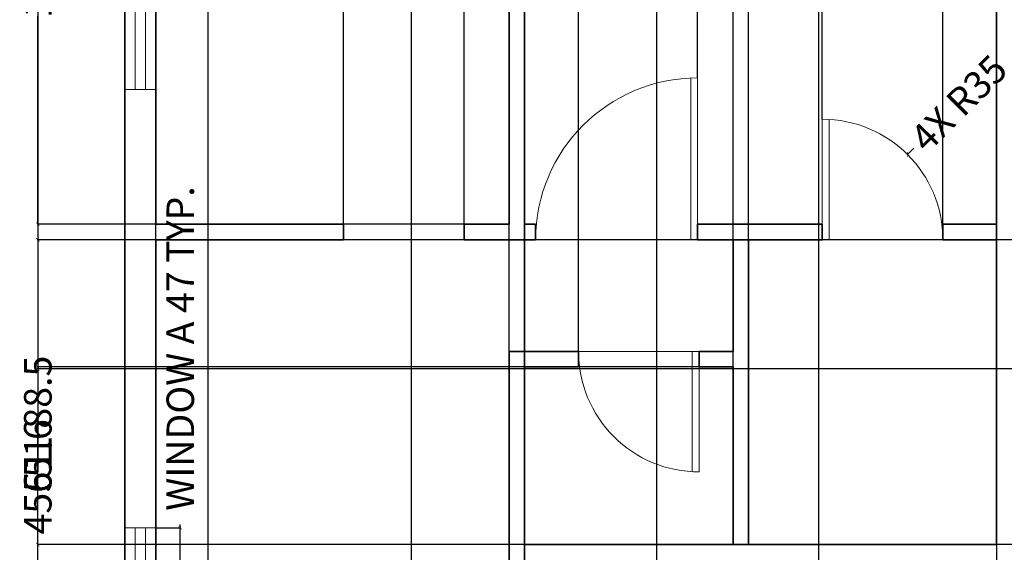
# Model space of a CAD drawing. Units: inches. Extents: x 878 to 1443, y 634 to 1188.
# Tile 2 of 5: x 878 to 1164, y 878 to 1033. Entities that reach past the tile are written whole.
import ezdxf

# ---------------------------------------------------------------- set-up
doc = ezdxf.new("R2010")
doc.units = ezdxf.units.IN
doc.header["$MEASUREMENT"] = 0
doc.layers.add('A-ANNO-DIMS', color=2, linetype='Continuous', lineweight=18)
doc.layers.add('A-WALL', color=7, linetype='Continuous', lineweight=35)
doc.layers.add('A-DOOR', color=41, linetype='Continuous', lineweight=18, true_color=0xf4ee51)
doc.layers.add('A-GLAZ', color=152, linetype='Continuous', lineweight=18, true_color=0x2776bb)
doc.styles.get("Standard").update_dxf_attribs({"font": 'arial.ttf'})
doc.dimstyles.get("Standard").update_dxf_attribs({"dimtxt": 8, "dimasz": 1, "dimexe": 0.18, "dimexo": 0.0625, "dimgap": 0.09, "dimtad": 0, "dimdec": 4, "dimzin": 0, "dimdsep": 46, "dimlunit": 3, "dimtxsty": 'Standard', "dimblk": 'ARCHTICK', "dimcen": 0.09, "dimclrd": 6, "dimclre": 5, "dimclrt": 140, "dimadec": 0, "dimazin": 0, "dimtfac": 1, "dimtdec": 4, "dimtofl": 0, "dimtmove": 0, "dimatfit": 3, "dimfxl": 1, "dimtolj": 1, "dimtzin": 0, "dimarcsym": 0})

# ---------------------------------------------------------------- blocks, each defined once
blk = doc.blocks.new('WIN-47IN')
for p, q in [((9, 47), (0, 47)), ((0, 47), (0, 0)), ((3, 0), (3, 47)), ((6, 0), (6, 47)), ((9, 0), (9, 47)), ((0, 0), (9, 0))]:
    blk.add_line(p, q)
blk = doc.blocks.new('DOOR-47IN')
for p, q in [((0, 47), (0, 0)), ((0, 2), (46.96, 2)), ((0, 0), (47, 0))]:
    blk.add_line(p, q)
blk.add_arc((0, 0), 47, 0, 90)
blk = doc.blocks.new('DOOR-35IN')
for p, q in [((0, 35), (0, 0)), ((2, 34.94), (2, 0)), ((0, 0), (35, 0))]:
    blk.add_line(p, q)
blk.add_arc((0, 0), 35, 360, 90)
blk = doc.blocks.new('_ArchTick')
at = {"color": 0, "linetype": 'ByBlock', "const_width": 0.15}
blk.add_lwpolyline([(-0.5, -0.5), (0.5, 0.5)], dxfattribs=at)
blk = doc.blocks.new('*D9')
at = {"layer": 'A-ANNO-DIMS', "color": 6, "lineweight": -2, "transparency": 16777216}
for p, q in [((924.95, 885.33), (924.95, 886.33)), ((924.95, 838.33), (924.95, 885.33))]:
    blk.add_line(p, q, dxfattribs=at)
at = {"layer": 'A-ANNO-DIMS', "color": 5, "lineweight": -2, "transparency": 16777216}
for p, q in [((917.96, 885.33), (925.13, 885.33)), ((917.96, 838.33), (925.13, 838.33))]:
    blk.add_line(p, q, dxfattribs=at)
at = {"layer": 'Defpoints', "color": 0, "lineweight": -2, "transparency": 16777216}
for p in [(917.9, 885.33), (924.95, 885.33), (917.9, 838.33)]:
    blk.add_point(p, dxfattribs=at)
at = {"layer": 'A-ANNO-DIMS', "color": 6, "lineweight": -2, "transparency": 16777216}
for p, rotation in [((924.95, 885.33), 90), ((924.95, 838.33), 270)]:
    blk.add_blockref('_ArchTick', p, dxfattribs=dict(at, rotation=rotation))
at = {"layer": 'A-ANNO-DIMS', "color": 140, "transparency": 16777216, "insert": (924.95, 937.4), "char_height": 8, "attachment_point": 5, "rotation": 90}
blk.add_mtext('\\A1;WINDOW A 47 TYP.', dxfattribs=at)
blk = doc.blocks.new('*D22')
at = {"layer": 'A-ANNO-DIMS', "color": 5, "lineweight": -2, "transparency": 16777216}
for p, q in [((908.84, 1120.47), (883.41, 1120.47)), ((908.84, 664.47), (883.41, 664.47))]:
    blk.add_line(p, q, dxfattribs=at)
at = {"layer": 'A-ANNO-DIMS', "color": 6, "lineweight": -2, "transparency": 16777216}
for p, q in [((883.59, 1120.47), (883.59, 901.56)), ((883.59, 664.47), (883.59, 883.38))]:
    blk.add_line(p, q, dxfattribs=at)
at = {"layer": 'Defpoints', "color": 0, "lineweight": -2, "transparency": 16777216}
for p in [(883.59, 1120.47), (908.9, 1120.47), (908.9, 664.47)]:
    blk.add_point(p, dxfattribs=at)
at = {"layer": 'A-ANNO-DIMS', "color": 6, "lineweight": -2, "transparency": 16777216}
for p, rotation in [((883.59, 1120.47), 90), ((883.59, 664.47), 270)]:
    blk.add_blockref('_ArchTick', p, dxfattribs=dict(at, rotation=rotation))
at = {"layer": 'A-ANNO-DIMS', "color": 140, "transparency": 16777216, "insert": (883.59, 892.47), "char_height": 8, "attachment_point": 5, "rotation": 90}
blk.add_mtext('\\A1;456', dxfattribs=at)
blk = doc.blocks.new('*D33')
at = {"layer": 'A-ANNO-DIMS', "color": 5, "lineweight": -2, "transparency": 16777216}
for p, q in [((917.9, 760.53), (917.9, 1145.96)), ((1020.4, 760.53), (1020.4, 1145.96))]:
    blk.add_line(p, q, dxfattribs=at)
at = {"layer": 'A-ANNO-DIMS', "color": 6, "lineweight": -2, "transparency": 16777216}
for p, q in [((917.9, 1145.78), (955.91, 1145.78)), ((1020.4, 1145.78), (982.39, 1145.78))]:
    blk.add_line(p, q, dxfattribs=at)
at = {"layer": 'Defpoints', "color": 0, "lineweight": -2, "transparency": 16777216}
for p in [(1020.4, 1145.78), (917.9, 760.47), (1020.4, 760.47)]:
    blk.add_point(p, dxfattribs=at)
at = {"layer": 'A-ANNO-DIMS', "color": 6, "lineweight": -2, "transparency": 16777216, "rotation": 180}
blk.add_blockref('_ArchTick', (917.9, 1145.78), dxfattribs=at)
at = {"layer": 'A-ANNO-DIMS', "color": 6, "lineweight": -2, "transparency": 16777216}
blk.add_blockref('_ArchTick', (1020.4, 1145.78), dxfattribs=at)
at = {"layer": 'A-ANNO-DIMS', "color": 140, "transparency": 16777216, "insert": (969.15, 1145.78), "char_height": 8, "attachment_point": 5}
blk.add_mtext('\\A1;102.5', dxfattribs=at)
blk = doc.blocks.new('*D34')
at = {"layer": 'A-ANNO-DIMS', "color": 5, "lineweight": -2, "transparency": 16777216}
for p, q in [((1024.9, 1111.41), (1024.9, 638.98)), ((1161.9, 1111.41), (1161.9, 638.98))]:
    blk.add_line(p, q, dxfattribs=at)
at = {"layer": 'A-ANNO-DIMS', "color": 6, "lineweight": -2, "transparency": 16777216}
for p, q in [((1024.9, 639.16), (1084.85, 639.16)), ((1161.9, 639.16), (1101.95, 639.16))]:
    blk.add_line(p, q, dxfattribs=at)
at = {"layer": 'Defpoints', "color": 0, "lineweight": -2, "transparency": 16777216}
for p in [(1024.9, 1111.47), (1161.9, 1111.47), (1161.9, 639.16)]:
    blk.add_point(p, dxfattribs=at)
at = {"layer": 'A-ANNO-DIMS', "color": 6, "lineweight": -2, "transparency": 16777216, "rotation": 180}
blk.add_blockref('_ArchTick', (1024.9, 639.16), dxfattribs=at)
at = {"layer": 'A-ANNO-DIMS', "color": 6, "lineweight": -2, "transparency": 16777216}
blk.add_blockref('_ArchTick', (1161.9, 639.16), dxfattribs=at)
at = {"layer": 'A-ANNO-DIMS', "color": 140, "transparency": 16777216, "insert": (1093.4, 639.16), "char_height": 8, "attachment_point": 5}
blk.add_mtext('\\A1;137', dxfattribs=at)
blk = doc.blocks.new('*D36')
at = {"layer": 'A-ANNO-DIMS', "color": 5, "lineweight": -2, "transparency": 16777216}
for p, q in [((1020.34, 1111.47), (883.41, 1111.47)), ((1020.34, 973.47), (883.41, 973.47))]:
    blk.add_line(p, q, dxfattribs=at)
at = {"layer": 'A-ANNO-DIMS', "color": 6, "lineweight": -2, "transparency": 16777216}
for p, q in [((883.59, 1111.47), (883.59, 1051.03)), ((883.59, 973.47), (883.59, 1033.91))]:
    blk.add_line(p, q, dxfattribs=at)
at = {"layer": 'Defpoints', "color": 0, "lineweight": -2, "transparency": 16777216}
for p in [(1020.4, 1111.47), (883.59, 973.47), (1020.4, 973.47)]:
    blk.add_point(p, dxfattribs=at)
at = {"layer": 'A-ANNO-DIMS', "color": 6, "lineweight": -2, "transparency": 16777216}
for p, rotation in [((883.59, 1111.47), 90), ((883.59, 973.47), 270)]:
    blk.add_blockref('_ArchTick', p, dxfattribs=dict(at, rotation=rotation))
at = {"layer": 'A-ANNO-DIMS', "color": 140, "transparency": 16777216, "insert": (883.59, 1042.47), "char_height": 8, "attachment_point": 5, "rotation": 90}
blk.add_mtext('\\A1;138', dxfattribs=at)
blk = doc.blocks.new('*D37')
at = {"layer": 'A-ANNO-DIMS', "color": 5, "lineweight": -2, "transparency": 16777216}
for p, q in [((1403.84, 968.97), (883.41, 968.97)), ((1403.84, 880.47), (883.41, 880.47))]:
    blk.add_line(p, q, dxfattribs=at)
at = {"layer": 'A-ANNO-DIMS', "color": 6, "lineweight": -2, "transparency": 16777216}
for p, q in [((883.59, 968.97), (883.59, 935.24)), ((883.59, 880.47), (883.59, 914.2))]:
    blk.add_line(p, q, dxfattribs=at)
at = {"layer": 'Defpoints', "color": 0, "lineweight": -2, "transparency": 16777216}
for p in [(1403.9, 968.97), (883.59, 880.47), (1403.9, 880.47)]:
    blk.add_point(p, dxfattribs=at)
at = {"layer": 'A-ANNO-DIMS', "color": 6, "lineweight": -2, "transparency": 16777216}
for p, rotation in [((883.59, 968.97), 90), ((883.59, 880.47), 270)]:
    blk.add_blockref('_ArchTick', p, dxfattribs=dict(at, rotation=rotation))
at = {"layer": 'A-ANNO-DIMS', "color": 140, "transparency": 16777216, "insert": (883.59, 924.72), "char_height": 8, "attachment_point": 5, "rotation": 90}
blk.add_mtext('\\A1;88.5', dxfattribs=at)
blk = doc.blocks.new('*D39')
at = {"layer": 'A-ANNO-DIMS', "color": 5, "lineweight": -2, "transparency": 16777216}
for p, q in [((1024.9, 880.53), (1024.9, 1145.96)), ((1085.4, 880.53), (1085.4, 1145.96))]:
    blk.add_line(p, q, dxfattribs=at)
at = {"layer": 'A-ANNO-DIMS', "color": 6, "lineweight": -2, "transparency": 16777216}
for p, q in [((1024.9, 1145.78), (1044.62, 1145.78)), ((1085.4, 1145.78), (1065.68, 1145.78))]:
    blk.add_line(p, q, dxfattribs=at)
at = {"layer": 'Defpoints', "color": 0, "lineweight": -2, "transparency": 16777216}
for p in [(1085.4, 1145.78), (1024.9, 880.47), (1085.4, 880.47)]:
    blk.add_point(p, dxfattribs=at)
at = {"layer": 'A-ANNO-DIMS', "color": 6, "lineweight": -2, "transparency": 16777216, "rotation": 180}
blk.add_blockref('_ArchTick', (1024.9, 1145.78), dxfattribs=at)
at = {"layer": 'A-ANNO-DIMS', "color": 6, "lineweight": -2, "transparency": 16777216}
blk.add_blockref('_ArchTick', (1085.4, 1145.78), dxfattribs=at)
at = {"layer": 'A-ANNO-DIMS', "color": 140, "transparency": 16777216, "insert": (1055.15, 1145.78), "char_height": 8, "attachment_point": 5}
blk.add_mtext('\\A1;60.5', dxfattribs=at)
blk = doc.blocks.new('*D40')
at = {"layer": 'A-ANNO-DIMS', "color": 5, "lineweight": -2, "transparency": 16777216}
for p, q in [((1089.9, 880.53), (1089.9, 1145.96)), ((1161.9, 880.53), (1161.9, 1145.96))]:
    blk.add_line(p, q, dxfattribs=at)
at = {"layer": 'A-ANNO-DIMS', "color": 6, "lineweight": -2, "transparency": 16777216}
for p, q in [((1089.9, 1145.78), (1120.15, 1145.78)), ((1161.9, 1145.78), (1131.64, 1145.78))]:
    blk.add_line(p, q, dxfattribs=at)
at = {"layer": 'Defpoints', "color": 0, "lineweight": -2, "transparency": 16777216}
for p in [(1161.9, 1145.78), (1089.9, 880.47), (1161.9, 880.47)]:
    blk.add_point(p, dxfattribs=at)
at = {"layer": 'A-ANNO-DIMS', "color": 6, "lineweight": -2, "transparency": 16777216, "rotation": 180}
blk.add_blockref('_ArchTick', (1089.9, 1145.78), dxfattribs=at)
at = {"layer": 'A-ANNO-DIMS', "color": 6, "lineweight": -2, "transparency": 16777216}
blk.add_blockref('_ArchTick', (1161.9, 1145.78), dxfattribs=at)
at = {"layer": 'A-ANNO-DIMS', "color": 140, "transparency": 16777216, "insert": (1125.9, 1145.78), "char_height": 8, "attachment_point": 5}
blk.add_mtext('\\A1;72', dxfattribs=at)
blk = doc.blocks.new('*D42')
at = {"layer": 'A-ANNO-DIMS', "color": 5, "lineweight": -2, "transparency": 16777216}
for p, q in [((1085.34, 932.07), (883.41, 932.07)), ((1085.34, 880.47), (883.41, 880.47))]:
    blk.add_line(p, q, dxfattribs=at)
at = {"layer": 'A-ANNO-DIMS', "color": 6, "lineweight": -2, "transparency": 16777216}
for p, q in [((883.59, 932.07), (883.59, 916.75)), ((883.59, 880.47), (883.59, 895.79))]:
    blk.add_line(p, q, dxfattribs=at)
at = {"layer": 'Defpoints', "color": 0, "lineweight": -2, "transparency": 16777216}
for p in [(883.59, 932.07), (1085.4, 932.07), (1085.4, 880.47)]:
    blk.add_point(p, dxfattribs=at)
at = {"layer": 'A-ANNO-DIMS', "color": 6, "lineweight": -2, "transparency": 16777216}
for p, rotation in [((883.59, 932.07), 90), ((883.59, 880.47), 270)]:
    blk.add_blockref('_ArchTick', p, dxfattribs=dict(at, rotation=rotation))
at = {"layer": 'A-ANNO-DIMS', "color": 140, "transparency": 16777216, "insert": (883.59, 906.27), "char_height": 8, "attachment_point": 5, "rotation": 90}
blk.add_mtext('\\A1;51.6', dxfattribs=at)
blk = doc.blocks.new('*D43')
at = {"layer": 'A-ANNO-DIMS', "color": 5, "lineweight": -2, "transparency": 16777216}
for p, q in [((1327.34, 931.47), (883.41, 931.47)), ((1327.34, 880.47), (883.41, 880.47))]:
    blk.add_line(p, q, dxfattribs=at)
at = {"layer": 'A-ANNO-DIMS', "color": 6, "lineweight": -2, "transparency": 16777216}
for p, q in [((883.59, 931.47), (883.59, 911.02)), ((883.59, 880.47), (883.59, 900.92))]:
    blk.add_line(p, q, dxfattribs=at)
at = {"layer": 'Defpoints', "color": 0, "lineweight": -2, "transparency": 16777216}
for p in [(883.59, 931.47), (1327.4, 931.47), (1327.4, 880.47)]:
    blk.add_point(p, dxfattribs=at)
at = {"layer": 'A-ANNO-DIMS', "color": 6, "lineweight": -2, "transparency": 16777216}
for p, rotation in [((883.59, 931.47), 90), ((883.59, 880.47), 270)]:
    blk.add_blockref('_ArchTick', p, dxfattribs=dict(at, rotation=rotation))
at = {"layer": 'A-ANNO-DIMS', "color": 140, "transparency": 16777216, "insert": (883.59, 905.97), "char_height": 8, "attachment_point": 5, "rotation": 90}
blk.add_mtext('\\A1;51', dxfattribs=at)
blk = doc.blocks.new('*D44')
at = {"layer": 'A-ANNO-DIMS', "color": 5, "lineweight": -2, "transparency": 16777216}
for p, q in [((917.9, 751.53), (917.9, 1145.96)), ((933.09, 751.53), (933.09, 1145.96))]:
    blk.add_line(p, q, dxfattribs=at)
at = {"layer": 'A-ANNO-DIMS', "color": 6, "lineweight": -2, "transparency": 16777216}
for p, q in [((917.9, 1145.78), (933.09, 1145.78)), ((933.09, 1145.78), (934.09, 1145.78))]:
    blk.add_line(p, q, dxfattribs=at)
at = {"layer": 'Defpoints', "color": 0, "lineweight": -2, "transparency": 16777216}
for p in [(933.09, 1145.78), (917.9, 751.47), (933.09, 751.47)]:
    blk.add_point(p, dxfattribs=at)
at = {"layer": 'A-ANNO-DIMS', "color": 6, "lineweight": -2, "transparency": 16777216, "rotation": 180}
blk.add_blockref('_ArchTick', (917.9, 1145.78), dxfattribs=at)
at = {"layer": 'A-ANNO-DIMS', "color": 6, "lineweight": -2, "transparency": 16777216}
blk.add_blockref('_ArchTick', (933.09, 1145.78), dxfattribs=at)
at = {"layer": 'A-ANNO-DIMS', "color": 140, "transparency": 16777216, "insert": (950.4, 1145.78), "char_height": 8, "attachment_point": 5}
blk.add_mtext('\\A1;15.187', dxfattribs=at)
blk = doc.blocks.new('*D45')
at = {"layer": 'A-ANNO-DIMS', "color": 5, "lineweight": -2, "transparency": 16777216}
for p, q in [((992.09, 751.53), (992.09, 1145.96)), ((1063.3, 751.53), (1063.3, 1145.96))]:
    blk.add_line(p, q, dxfattribs=at)
at = {"layer": 'A-ANNO-DIMS', "color": 6, "lineweight": -2, "transparency": 16777216}
for p, q in [((992.09, 1145.78), (1014.18, 1145.78)), ((1063.3, 1145.78), (1041.21, 1145.78))]:
    blk.add_line(p, q, dxfattribs=at)
at = {"layer": 'Defpoints', "color": 0, "lineweight": -2, "transparency": 16777216}
for p in [(1063.3, 1145.78), (992.09, 751.47), (1063.3, 751.47)]:
    blk.add_point(p, dxfattribs=at)
at = {"layer": 'A-ANNO-DIMS', "color": 6, "lineweight": -2, "transparency": 16777216, "rotation": 180}
blk.add_blockref('_ArchTick', (992.09, 1145.78), dxfattribs=at)
at = {"layer": 'A-ANNO-DIMS', "color": 6, "lineweight": -2, "transparency": 16777216}
blk.add_blockref('_ArchTick', (1063.3, 1145.78), dxfattribs=at)
at = {"layer": 'A-ANNO-DIMS', "color": 140, "transparency": 16777216, "insert": (1027.69, 1145.78), "char_height": 8, "attachment_point": 5}
blk.add_mtext('\\A1;71.22', dxfattribs=at)
blk = doc.blocks.new('*D46')
at = {"layer": 'A-ANNO-DIMS', "color": 5, "lineweight": -2, "transparency": 16777216}
for p, q in [((1110.3, 751.53), (1110.3, 1145.96)), ((1172.39, 751.53), (1172.39, 1145.96))]:
    blk.add_line(p, q, dxfattribs=at)
at = {"layer": 'A-ANNO-DIMS', "color": 6, "lineweight": -2, "transparency": 16777216}
for p, q in [((1110.3, 1145.78), (1127.73, 1145.78)), ((1172.39, 1145.78), (1154.96, 1145.78))]:
    blk.add_line(p, q, dxfattribs=at)
at = {"layer": 'Defpoints', "color": 0, "lineweight": -2, "transparency": 16777216}
for p in [(1172.39, 1145.78), (1110.3, 751.47), (1172.39, 751.47)]:
    blk.add_point(p, dxfattribs=at)
at = {"layer": 'A-ANNO-DIMS', "color": 6, "lineweight": -2, "transparency": 16777216, "rotation": 180}
blk.add_blockref('_ArchTick', (1110.3, 1145.78), dxfattribs=at)
at = {"layer": 'A-ANNO-DIMS', "color": 6, "lineweight": -2, "transparency": 16777216}
blk.add_blockref('_ArchTick', (1172.39, 1145.78), dxfattribs=at)
at = {"layer": 'A-ANNO-DIMS', "color": 140, "transparency": 16777216, "insert": (1141.35, 1145.78), "char_height": 8, "attachment_point": 5}
blk.add_mtext('\\A1;62.08', dxfattribs=at)
blk = doc.blocks.new('*D49')
at = {"layer": 'A-ANNO-DIMS', "color": 5, "lineweight": -2, "transparency": 16777216}
for p, q in [((917.9, 973.53), (917.9, 1145.96)), ((972.37, 973.53), (972.37, 1145.96))]:
    blk.add_line(p, q, dxfattribs=at)
at = {"layer": 'A-ANNO-DIMS', "color": 6, "lineweight": -2, "transparency": 16777216}
for p, q in [((917.9, 1145.78), (931.54, 1145.78)), ((972.37, 1145.78), (958.72, 1145.78))]:
    blk.add_line(p, q, dxfattribs=at)
at = {"layer": 'Defpoints', "color": 0, "lineweight": -2, "transparency": 16777216}
for p in [(972.37, 1145.78), (917.9, 973.47), (972.37, 973.47)]:
    blk.add_point(p, dxfattribs=at)
at = {"layer": 'A-ANNO-DIMS', "color": 6, "lineweight": -2, "transparency": 16777216, "rotation": 180}
blk.add_blockref('_ArchTick', (917.9, 1145.78), dxfattribs=at)
at = {"layer": 'A-ANNO-DIMS', "color": 6, "lineweight": -2, "transparency": 16777216}
blk.add_blockref('_ArchTick', (972.37, 1145.78), dxfattribs=at)
at = {"layer": 'A-ANNO-DIMS', "color": 140, "transparency": 16777216, "insert": (945.13, 1145.78), "char_height": 8, "attachment_point": 5}
blk.add_mtext('\\A1;54.47', dxfattribs=at)
blk = doc.blocks.new('*D50')
at = {"layer": 'A-ANNO-DIMS', "color": 5, "lineweight": -2, "transparency": 16777216}
for p, q in [((972.37, 973.53), (972.37, 1145.96)), ((1007.37, 973.53), (1007.37, 1145.96))]:
    blk.add_line(p, q, dxfattribs=at)
at = {"layer": 'A-ANNO-DIMS', "color": 6, "lineweight": -2, "transparency": 16777216}
for p, q in [((972.37, 1145.78), (984.02, 1145.78)), ((1007.37, 1145.78), (995.71, 1145.78))]:
    blk.add_line(p, q, dxfattribs=at)
at = {"layer": 'Defpoints', "color": 0, "lineweight": -2, "transparency": 16777216}
for p in [(1007.37, 1145.78), (972.37, 973.47), (1007.37, 973.47)]:
    blk.add_point(p, dxfattribs=at)
at = {"layer": 'A-ANNO-DIMS', "color": 6, "lineweight": -2, "transparency": 16777216, "rotation": 180}
blk.add_blockref('_ArchTick', (972.37, 1145.78), dxfattribs=at)
at = {"layer": 'A-ANNO-DIMS', "color": 6, "lineweight": -2, "transparency": 16777216}
blk.add_blockref('_ArchTick', (1007.37, 1145.78), dxfattribs=at)
at = {"layer": 'A-ANNO-DIMS', "color": 140, "transparency": 16777216, "insert": (989.87, 1145.78), "char_height": 8, "attachment_point": 5}
blk.add_mtext('\\A1;35', dxfattribs=at)
blk = doc.blocks.new('*D52')
at = {"layer": 'A-ANNO-DIMS', "color": 6, "lineweight": -2, "transparency": 16777216}
for p, q in [((1146.32, 1145.78), (1145.32, 1145.78)), ((1161.9, 1145.78), (1146.32, 1145.78))]:
    blk.add_line(p, q, dxfattribs=at)
at = {"layer": 'A-ANNO-DIMS', "color": 5, "lineweight": -2, "transparency": 16777216}
for p, q in [((1146.32, 973.53), (1146.32, 1145.96)), ((1161.9, 973.53), (1161.9, 1145.96))]:
    blk.add_line(p, q, dxfattribs=at)
at = {"layer": 'Defpoints', "color": 0, "lineweight": -2, "transparency": 16777216}
for p in [(1146.32, 1145.78), (1146.32, 973.47), (1161.9, 973.47)]:
    blk.add_point(p, dxfattribs=at)
at = {"layer": 'A-ANNO-DIMS', "color": 6, "lineweight": -2, "transparency": 16777216, "rotation": 180}
blk.add_blockref('_ArchTick', (1146.32, 1145.78), dxfattribs=at)
at = {"layer": 'A-ANNO-DIMS', "color": 6, "lineweight": -2, "transparency": 16777216}
blk.add_blockref('_ArchTick', (1161.9, 1145.78), dxfattribs=at)
at = {"layer": 'A-ANNO-DIMS', "color": 140, "transparency": 16777216, "insert": (1132.1, 1145.78), "char_height": 8, "attachment_point": 5}
blk.add_mtext('\\A1;15.58', dxfattribs=at)
blk = doc.blocks.new('*D53')
at = {"layer": 'A-ANNO-DIMS', "color": 5, "lineweight": -2, "transparency": 16777216}
for p, q in [((1075.11, 1016.03), (1075.11, 1145.96)), ((1111.32, 1004.03), (1111.32, 1145.96))]:
    blk.add_line(p, q, dxfattribs=at)
at = {"layer": 'A-ANNO-DIMS', "color": 6, "lineweight": -2, "transparency": 16777216}
for p, q in [((1075.11, 1145.78), (1080.4, 1145.78)), ((1111.32, 1145.78), (1106.03, 1145.78))]:
    blk.add_line(p, q, dxfattribs=at)
at = {"layer": 'Defpoints', "color": 0, "lineweight": -2, "transparency": 16777216}
for p in [(1111.32, 1145.78), (1075.11, 1015.97), (1111.32, 1003.97)]:
    blk.add_point(p, dxfattribs=at)
at = {"layer": 'A-ANNO-DIMS', "color": 6, "lineweight": -2, "transparency": 16777216, "rotation": 180}
blk.add_blockref('_ArchTick', (1075.11, 1145.78), dxfattribs=at)
at = {"layer": 'A-ANNO-DIMS', "color": 6, "lineweight": -2, "transparency": 16777216}
blk.add_blockref('_ArchTick', (1111.32, 1145.78), dxfattribs=at)
at = {"layer": 'A-ANNO-DIMS', "color": 140, "transparency": 16777216, "insert": (1093.21, 1145.78), "char_height": 8, "attachment_point": 5}
blk.add_mtext('\\A1;36.21', dxfattribs=at)
blk = doc.blocks.new('*D56')
at = {"layer": 'A-ANNO-DIMS', "color": 5, "lineweight": -2, "transparency": 16777216}
for p, q in [((1020.4, 936.63), (1020.4, 1145.96)), ((1040.54, 936.63), (1040.54, 1145.96))]:
    blk.add_line(p, q, dxfattribs=at)
at = {"layer": 'A-ANNO-DIMS', "color": 6, "lineweight": -2, "transparency": 16777216}
for p, q in [((1020.4, 1145.78), (1040.54, 1145.78)), ((1040.54, 1145.78), (1041.54, 1145.78))]:
    blk.add_line(p, q, dxfattribs=at)
at = {"layer": 'Defpoints', "color": 0, "lineweight": -2, "transparency": 16777216}
for p in [(1040.54, 1145.78), (1020.4, 936.57), (1040.54, 936.57)]:
    blk.add_point(p, dxfattribs=at)
at = {"layer": 'A-ANNO-DIMS', "color": 6, "lineweight": -2, "transparency": 16777216, "rotation": 180}
blk.add_blockref('_ArchTick', (1020.4, 1145.78), dxfattribs=at)
at = {"layer": 'A-ANNO-DIMS', "color": 6, "lineweight": -2, "transparency": 16777216}
blk.add_blockref('_ArchTick', (1040.54, 1145.78), dxfattribs=at)
at = {"layer": 'A-ANNO-DIMS', "color": 140, "transparency": 16777216, "insert": (1055.18, 1145.78), "char_height": 8, "attachment_point": 5}
blk.add_mtext('\\A1;20.14', dxfattribs=at)
blk = doc.blocks.new('*D63')
at = {"layer": 'A-ANNO-DIMS', "color": 5, "lineweight": -2, "transparency": 16777216}
for p, q in [((1020.4, 851.67), (1020.4, 1145.96)), ((1024.9, 851.67), (1024.9, 1145.96))]:
    blk.add_line(p, q, dxfattribs=at)
at = {"layer": 'A-ANNO-DIMS', "color": 6, "lineweight": -2, "transparency": 16777216}
for p, q in [((1020.4, 1145.78), (1024.9, 1145.78)), ((1024.9, 1145.78), (1025.9, 1145.78))]:
    blk.add_line(p, q, dxfattribs=at)
at = {"layer": 'Defpoints', "color": 0, "lineweight": -2, "transparency": 16777216}
for p in [(1024.9, 1145.78), (1020.4, 851.61), (1024.9, 851.61)]:
    blk.add_point(p, dxfattribs=at)
at = {"layer": 'A-ANNO-DIMS', "color": 6, "lineweight": -2, "transparency": 16777216, "rotation": 180}
blk.add_blockref('_ArchTick', (1020.4, 1145.78), dxfattribs=at)
at = {"layer": 'A-ANNO-DIMS', "color": 6, "lineweight": -2, "transparency": 16777216}
blk.add_blockref('_ArchTick', (1024.9, 1145.78), dxfattribs=at)
at = {"layer": 'A-ANNO-DIMS', "color": 140, "transparency": 16777216, "insert": (1033.46, 1145.78), "char_height": 8, "attachment_point": 5}
blk.add_mtext('\\A1;4.5', dxfattribs=at)
blk = doc.blocks.new('*D70')
at = {"layer": 'A-ANNO-DIMS', "color": 6, "lineweight": -2, "transparency": 16777216}
blk.add_line((1137.88, 995.53), (1136.07, 993.72), dxfattribs=at)
at = {"layer": 'A-ANNO-DIMS', "color": 5, "lineweight": -2, "transparency": 16777216}
for p, q in [((1111.23, 968.97), (1111.41, 968.97)), ((1111.32, 968.88), (1111.32, 969.06))]:
    blk.add_line(p, q, dxfattribs=at)
at = {"layer": 'Defpoints', "color": 0, "lineweight": -2, "transparency": 16777216}
for p in [(1136.07, 993.72), (1111.32, 968.97)]:
    blk.add_point(p, dxfattribs=at)
at = {"layer": 'A-ANNO-DIMS', "color": 6, "lineweight": -2, "transparency": 16777216, "rotation": 224.9999525404688}
blk.add_blockref('_ArchTick', (1136.07, 993.72), dxfattribs=at)
at = {"layer": 'A-ANNO-DIMS', "color": 140, "transparency": 16777216, "insert": (1150.92, 1008.57), "char_height": 8, "attachment_point": 5, "rotation": 45}
blk.add_mtext('\\A1;4X R35', dxfattribs=at)

msp = doc.modelspace()

# ---------------------------------------------------------------- linework, layer by layer
at = {"layer": 'A-WALL'}
for p, q in [((908.8987, 664.4702), (908.8987, 1120.4702)), ((917.8987, 973.4702), (917.8987, 1111.4702)), ((1020.3987, 1111.4702), (1020.3987, 973.4702)), ((1024.8987, 1111.4702), (1024.8987, 973.4702)), ((1161.8987, 1111.4702), (1161.8987, 973.4702)), ((972.3652, 973.4702), (917.8987, 973.4702)), ((972.3652, 968.9702), (972.3652, 973.4702)), ((1020.3987, 973.4702), (1007.3652, 973.4702)), ((1007.3652, 968.9702), (1007.3652, 973.4702)), ((1028.1079, 973.4702), (1024.8987, 973.4702)), ((1028.1079, 968.9702), (1028.1079, 973.4702)), ((1111.3192, 973.4702), (1075.1079, 973.4702)), ((1075.1079, 968.9702), (1075.1079, 973.4702)), ((1111.3192, 968.9702), (1111.3192, 973.4702)), ((1161.8987, 973.4702), (1146.3192, 973.4702)), ((1146.3192, 968.9702), (1146.3192, 973.4702)), ((917.8987, 760.4702), (917.8987, 968.9702)), ((972.3652, 968.9702), (917.8987, 968.9702)), ((1020.3987, 968.9702), (1007.3652, 968.9702)), ((1028.1079, 968.9702), (1020.3987, 968.9702)), ((1111.3192, 968.9702), (1075.1079, 968.9702)), ((1085.3987, 968.9702), (1085.3987, 936.5702)), ((1089.8987, 968.9702), (1089.8987, 880.4702)), ((1161.8987, 968.9702), (1146.3192, 968.9702)), ((1161.8987, 968.9702), (1161.8987, 880.4702)), ((1020.3987, 936.5702), (1020.3987, 851.6074)), ((1040.5379, 936.5702), (1020.3987, 936.5702)), ((1040.5379, 936.5702), (1040.5379, 932.0702)), ((1085.3987, 936.5702), (1075.5379, 936.5702)), ((1075.5379, 936.5702), (1075.5379, 932.0702)), ((1024.8987, 932.0702), (1024.8987, 880.4702)), ((1040.5379, 932.0702), (1024.8987, 932.0702)), ((1085.3987, 932.0702), (1075.5379, 932.0702)), ((1085.3987, 932.0702), (1085.3987, 880.4702)), ((1161.8987, 880.4702), (1024.8987, 880.4702))]:
    msp.add_line(p, q, dxfattribs=at)

# ---------------------------------------------------------------- block references
at = {"layer": 'A-DOOR'}
for name, p, rotation in [('DOOR-47IN', (1075.1079, 968.9702), 90.00000000000021), ('DOOR-35IN', (1075.5379, 936.5702), 180)]:
    msp.add_blockref(name, p, dxfattribs=dict(at, rotation=rotation))
msp.add_blockref('DOOR-35IN', (1111.3192, 968.9702), dxfattribs=at)
at = {"layer": 'A-GLAZ'}
for p in [(908.8987, 1012.5982), (908.8987, 838.3253)]:
    msp.add_blockref('WIN-47IN', p, dxfattribs=at)

# ---------------------------------------------------------------- dimensions: what is measured, and where the dimension line sits
at = {"layer": 'A-ANNO-DIMS'}
for base, p1, p2, override, picture, middle in [((1020.3987, 1145.7802), (917.8987, 760.4702), (1020.3987, 760.4702), {"dimdec": 1, "dimlfac": 1, "dimrnd": 0, "dimzin": 0, "dimdsep": 46, "dimlunit": 2}, '*D33', (969.1487, 1145.7802)), ((933.0853, 1145.7802), (917.8987, 751.4702), (933.0853, 751.4702), {"dimdec": 3, "dimlfac": 1, "dimrnd": 0, "dimzin": 0, "dimdsep": 46, "dimlunit": 2}, '*D44', (950.4045, 1145.7802)), ((972.3652, 1145.7802), (917.8987, 973.4702), (972.3652, 973.4702), {"dimdec": 2, "dimlfac": 1, "dimrnd": 0, "dimzin": 0, "dimdsep": 46, "dimlunit": 2}, '*D49', (945.1319, 1145.7802)), ((1007.3652, 1145.7802), (972.3652, 973.4702), (1007.3652, 973.4702), {"dimdec": 0, "dimlfac": 1, "dimrnd": 0, "dimzin": 0, "dimdsep": 46, "dimlunit": 2}, '*D50', (989.8652, 1145.7802)), ((1063.3038, 1145.7802), (992.0853, 751.4702), (1063.3038, 751.4702), {"dimdec": 2, "dimlfac": 1, "dimrnd": 0, "dimzin": 0, "dimdsep": 46, "dimlunit": 2}, '*D45', (1027.6946, 1145.7802)), ((1040.5379, 1145.7802), (1020.3987, 936.5702), (1040.5379, 936.5702), {"dimdec": 2, "dimlfac": 1, "dimrnd": 0, "dimzin": 0, "dimdsep": 46, "dimlunit": 2}, '*D56', (1055.1777, 1145.7802)), ((1024.8987, 1145.7802), (1020.3987, 851.6074), (1024.8987, 851.6074), {"dimdec": 1, "dimlfac": 1, "dimrnd": 0, "dimzin": 0, "dimdsep": 46, "dimlunit": 2}, '*D63', (1033.462, 1145.7802)), ((1085.3987, 1145.7802), (1024.8987, 880.4702), (1085.3987, 880.4702), {"dimdec": 1, "dimlfac": 1, "dimrnd": 0, "dimzin": 0, "dimdsep": 46, "dimlunit": 2}, '*D39', (1055.1487, 1145.7802)), ((1111.3192, 1145.7802), (1075.1079, 1015.9702), (1111.3192, 1003.9702), {"dimdec": 2, "dimlfac": 1, "dimrnd": 0, "dimzin": 0, "dimdsep": 46, "dimlunit": 2}, '*D53', (1093.2135, 1145.7802)), ((1161.8987, 1145.7802), (1089.8987, 880.4702), (1161.8987, 880.4702), {"dimdec": 0, "dimlfac": 1, "dimrnd": 0, "dimzin": 0, "dimdsep": 46, "dimlunit": 2}, '*D40', (1125.8987, 1145.7802)), ((1172.3876, 1145.7802), (1110.3038, 751.4702), (1172.3876, 751.4702), {"dimdec": 2, "dimlfac": 1, "dimrnd": 0, "dimzin": 0, "dimdsep": 46, "dimlunit": 2}, '*D46', (1141.3457, 1145.7802)), ((1146.3192, 1145.7802), (1161.8987, 973.4702), (1146.3192, 973.4702), {"dimdec": 2, "dimlfac": 1, "dimrnd": 0, "dimzin": 0, "dimdsep": 46, "dimlunit": 2}, '*D52', (1132.0996, 1145.7802)), ((1161.8987, 639.1602), (1024.8987, 1111.4702), (1161.8987, 1111.4702), {"dimdec": 0, "dimlfac": 1, "dimrnd": 0, "dimzin": 0, "dimdsep": 46, "dimlunit": 2}, '*D34', (1093.3987, 639.1602))]:
    dim = msp.add_linear_dim(base=base, p1=p1, p2=p2, dimstyle='Standard', override=override, dxfattribs=at)
    dim.commit()
    dim.dimension.update_dxf_attribs({"geometry": picture, "text_midpoint": middle})
for base, p1, p2, override, picture, middle in [((883.5887, 1120.4702), (908.8987, 664.4702), (908.8987, 1120.4702), {"dimdec": 0, "dimlfac": 1, "dimrnd": 0, "dimzin": 0, "dimdsep": 46, "dimlunit": 2}, '*D22', (883.5887, 892.4702)), ((883.5887, 973.4702), (1020.3987, 1111.4702), (1020.3987, 973.4702), {"dimdec": 0, "dimlfac": 1, "dimrnd": 0, "dimzin": 0, "dimdsep": 46, "dimlunit": 2}, '*D36', (883.5887, 1042.4702)), ((883.5887, 880.4702), (1403.8987, 968.9702), (1403.8987, 880.4702), {"dimdec": 1, "dimlfac": 1, "dimrnd": 0, "dimzin": 0, "dimdsep": 46, "dimlunit": 2}, '*D37', (883.5887, 924.7202)), ((883.5887, 932.0702), (1085.3987, 880.4702), (1085.3987, 932.0702), {"dimdec": 1, "dimlfac": 1, "dimrnd": 0, "dimzin": 0, "dimdsep": 46, "dimlunit": 2}, '*D42', (883.5887, 906.2702)), ((883.5887, 931.4702), (1327.3987, 880.4702), (1327.3987, 931.4702), {"dimdec": 0, "dimlfac": 1, "dimrnd": 0, "dimzin": 0, "dimdsep": 46, "dimlunit": 2}, '*D43', (883.5887, 905.9702))]:
    dim = msp.add_linear_dim(base=base, p1=p1, p2=p2, angle=90, dimstyle='Standard', override=override, dxfattribs=at)
    dim.commit()
    dim.dimension.update_dxf_attribs({"geometry": picture, "text_midpoint": middle})
dim = msp.add_radius_dim(center=(1111.3192, 968.9702), mpoint=(1136.0679, 993.7189), text='4X <>', dimstyle='Standard', override={"dimdec": 0, "dimlfac": 1, "dimrnd": 0, "dimzin": 0, "dimdsep": 46, "dimlunit": 2}, dxfattribs=at)
dim.commit()
dim.dimension.update_dxf_attribs({"geometry": '*D70', "text_midpoint": (1150.9172, 1008.5681), "dimtype": 164})
dim = msp.add_linear_dim(base=(924.9487, 885.3253), p1=(917.8987, 838.3253), p2=(917.8987, 885.3253), angle=90, text='WINDOW A <> TYP.', dimstyle='Standard', override={"dimdec": 0, "dimlfac": 1, "dimrnd": 0, "dimzin": 0, "dimdsep": 46, "dimlunit": 2}, dxfattribs=at)
dim.commit()
dim.dimension.update_dxf_attribs({"geometry": '*D9', "text_midpoint": (924.9487, 937.4003)})

doc.saveas('drawing.dxf')
